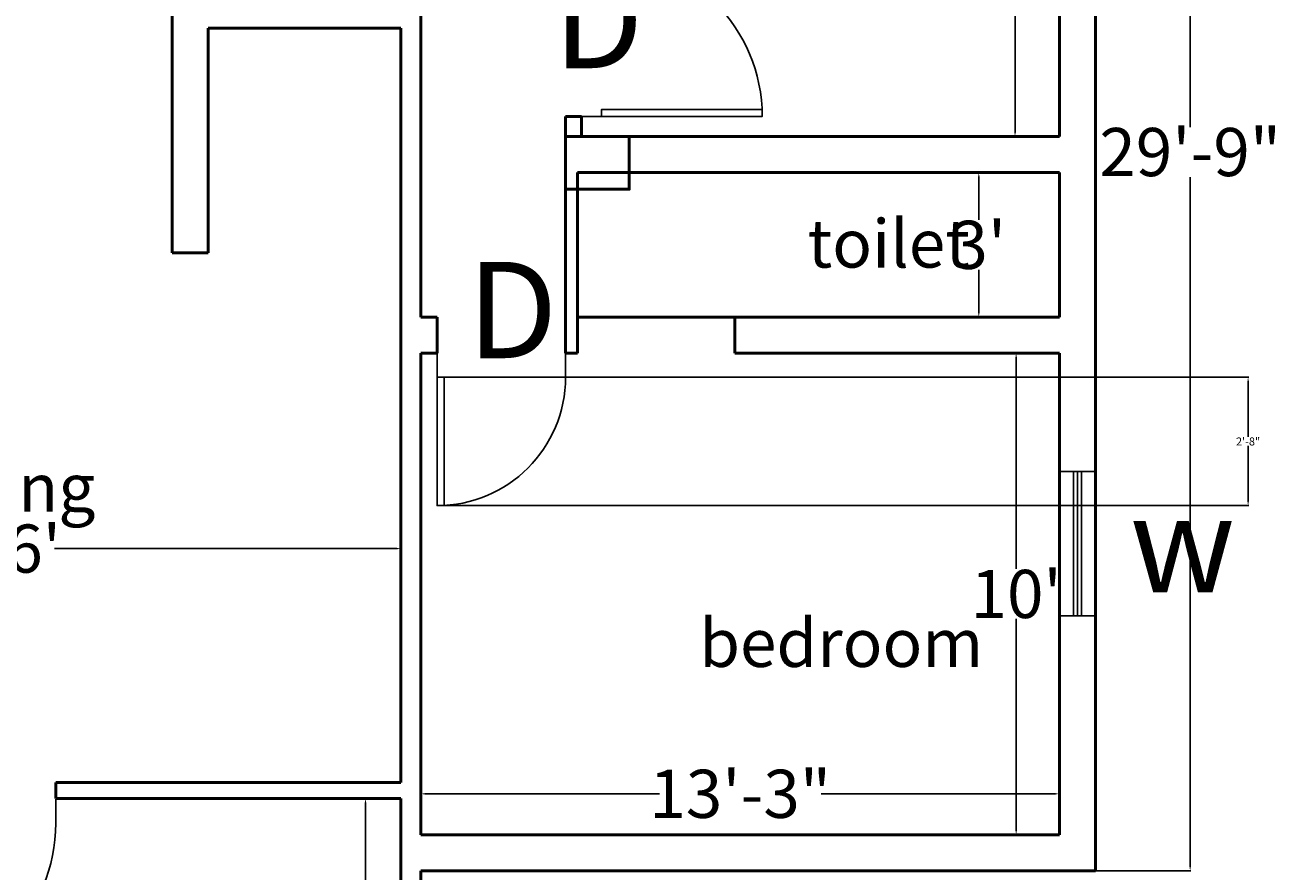
# Model space of a CAD drawing. Units: inches. Extents: x 409 to 7572, y 7 to 725.
# Tile 32 of 38: x 5952 to 6263, y 315 to 526. Entities that reach past the tile are written whole.
import ezdxf

# ---------------------------------------------------------------- set-up
doc = ezdxf.new("R2010")
doc.units = ezdxf.units.IN
doc.header["$MEASUREMENT"] = 0
for name, color, linetype, lineweight in [('A-ANNO-DIMS', 2, 'Continuous', 18), ('A-ANNO-SYMB', 3, 'Continuous', 25), ('A-AREA-IDEN', 7, 'Continuous', 25), ('A-DOOR', 3, 'Continuous', 25), ('A-GLAZ', 4, 'Continuous', 25), ('A-WALL', 7, 'Continuous', 50)]:
    doc.layers.add(name, color=color, linetype=linetype, lineweight=lineweight)
doc.styles.get("Standard").update_dxf_attribs({"font": 'arial.ttf'})
doc.dimstyles.get("Standard").update_dxf_attribs({"dimtxt": 2, "dimasz": 1, "dimexe": 0.18, "dimexo": 0.0625, "dimgap": 0.09, "dimtad": 0, "dimtih": 1, "dimtoh": 1, "dimdec": 0, "dimzin": 0, "dimdsep": 46, "dimlunit": 3, "dimtxsty": 'Standard', "dimcen": 0.09, "dimadec": 0, "dimazin": 0, "dimtfac": 1, "dimtdec": 0, "dimtofl": 0, "dimtmove": 0, "dimatfit": 3, "dimfxl": 1, "dimtolj": 1, "dimtzin": 0, "dimarcsym": 0})

# ---------------------------------------------------------------- blocks, each defined once
blk = doc.blocks.new('*U5')
for p, q in [((0, 0), (0, 6)), ((40, 0), (40, 6))]:
    blk.add_line(p, q)
blk.add_lwpolyline([(0, 0), (0, -40), (1.75, -40), (1.75, 0)], close=True)
blk.add_arc((0, 0), 40, 270, 0)
blk = doc.blocks.new('*U6')
for p, q in [((0, 0), (0, -6)), ((-40, 0), (-40, -6))]:
    blk.add_line(p, q)
blk.add_lwpolyline([(0, 0), (0, 40), (-1.75, 40), (-1.75, 0)], close=True)
blk.add_arc((0, 0), 40, 90, 180)
blk = doc.blocks.new('*U7')
for p, q in [((0, 0), (0, 6)), ((32, 0), (32, 6))]:
    blk.add_line(p, q)
blk.add_lwpolyline([(0, 0), (0, -32), (1.75, -32), (1.75, 0)], close=True)
blk.add_arc((0, 0), 32, 270, 0)
blk = doc.blocks.new('*D130')
at = {"layer": 'A-ANNO-DIMS', "color": 0, "lineweight": -2, "transparency": 16777216}
for p, q in [((6209.72, 618.53), (6198.55, 618.53)), ((6198.73, 617.53), (6198.73, 564.75)), ((6198.73, 499.53), (6198.73, 552.31)), ((6209.72, 498.53), (6198.55, 498.53))]:
    blk.add_line(p, q, dxfattribs=at)
at = {"layer": 'A-ANNO-DIMS', "color": 0, "transparency": 16777216}
for points in [[(6198.57, 617.53), (6198.9, 617.53), (6198.73, 618.53)], [(6198.57, 499.53), (6198.9, 499.53), (6198.73, 498.53)]]:
    blk.add_solid(points, dxfattribs=at)
at = {"layer": 'DEFPOINTS', "color": 0, "transparency": 16777216}
for p in [(6198.73, 618.53), (6209.78, 618.53), (6209.78, 498.53)]:
    blk.add_point(p, dxfattribs=at)
at = {"layer": 'A-ANNO-DIMS', "color": 0, "transparency": 16777216, "insert": (6198.73, 558.53), "char_height": 2, "attachment_point": 5}
blk.add_mtext("\\A1;{\\H6x;10'}", dxfattribs=at)
blk = doc.blocks.new('*D131')
at = {"layer": 'A-ANNO-DIMS', "color": 0, "lineweight": -2, "transparency": 16777216}
for p, q in [((6209.72, 444.53), (6198.84, 444.53)), ((6199.02, 443.53), (6199.02, 390.75)), ((6199.02, 325.53), (6199.02, 378.31)), ((6209.72, 324.53), (6198.84, 324.53))]:
    blk.add_line(p, q, dxfattribs=at)
at = {"layer": 'A-ANNO-DIMS', "color": 0, "transparency": 16777216}
for points in [[(6198.85, 443.53), (6199.18, 443.53), (6199.02, 444.53)], [(6198.85, 325.53), (6199.18, 325.53), (6199.02, 324.53)]]:
    blk.add_solid(points, dxfattribs=at)
at = {"layer": 'DEFPOINTS', "color": 0, "transparency": 16777216}
for p in [(6199.02, 444.53), (6209.78, 444.53), (6209.78, 324.53)]:
    blk.add_point(p, dxfattribs=at)
at = {"layer": 'A-ANNO-DIMS', "color": 0, "transparency": 16777216, "insert": (6199.02, 384.53), "char_height": 2, "attachment_point": 5}
blk.add_mtext("\\A1;{\\H6x;10'}", dxfattribs=at)
blk = doc.blocks.new('*D122')
at = {"layer": 'A-ANNO-DIMS', "color": 0, "lineweight": -2, "transparency": 16777216}
for p, q in [((6050.78, 324.59), (6050.78, 334.9)), ((6051.78, 334.72), (6110.15, 334.72)), ((6208.78, 334.72), (6150.42, 334.72)), ((6209.78, 324.59), (6209.78, 334.9))]:
    blk.add_line(p, q, dxfattribs=at)
at = {"layer": 'A-ANNO-DIMS', "color": 0, "transparency": 16777216}
for points in [[(6051.78, 334.88), (6051.78, 334.55), (6050.78, 334.72)], [(6208.78, 334.88), (6208.78, 334.55), (6209.78, 334.72)]]:
    blk.add_solid(points, dxfattribs=at)
at = {"layer": 'DEFPOINTS', "color": 0, "transparency": 16777216}
for p in [(6050.78, 334.72), (6050.78, 324.53), (6209.78, 324.53)]:
    blk.add_point(p, dxfattribs=at)
at = {"layer": 'A-ANNO-DIMS', "color": 0, "transparency": 16777216, "insert": (6130.28, 334.72), "char_height": 2, "attachment_point": 5}
blk.add_mtext('\\A1;{\\H6x;13\'-3"}', dxfattribs=at)
blk = doc.blocks.new('*D123')
at = {"layer": 'A-ANNO-DIMS', "color": 0, "lineweight": -2, "transparency": 16777216}
for p, q in [((6045.72, 333.53), (6036.79, 333.53)), ((6036.97, 332.53), (6036.97, 255.65)), ((6036.97, 166.53), (6036.97, 243.42)), ((6045.72, 165.53), (6036.79, 165.53))]:
    blk.add_line(p, q, dxfattribs=at)
at = {"layer": 'A-ANNO-DIMS', "color": 0, "transparency": 16777216}
for points in [[(6036.8, 332.53), (6037.14, 332.53), (6036.97, 333.53)], [(6036.8, 166.53), (6037.14, 166.53), (6036.97, 165.53)]]:
    blk.add_solid(points, dxfattribs=at)
at = {"layer": 'DEFPOINTS', "color": 0, "transparency": 16777216}
for p in [(6045.78, 333.53), (6036.97, 165.53), (6045.78, 165.53)]:
    blk.add_point(p, dxfattribs=at)
at = {"layer": 'A-ANNO-DIMS', "color": 0, "transparency": 16777216, "insert": (6036.97, 249.53), "char_height": 2, "attachment_point": 5}
blk.add_mtext("\\A1;{\\H6x;14'}", dxfattribs=at)
blk = doc.blocks.new('*D136')
at = {"layer": 'A-ANNO-DIMS', "color": 0, "lineweight": -2, "transparency": 16777216}
for p, q in [((5853.78, 403.47), (5853.78, 395.65)), ((6045.78, 403.47), (6045.78, 395.65)), ((5854.78, 395.83), (5940.08, 395.83)), ((6044.78, 395.83), (5959.49, 395.83))]:
    blk.add_line(p, q, dxfattribs=at)
at = {"layer": 'A-ANNO-DIMS', "color": 0, "transparency": 16777216}
for points in [[(5854.78, 396), (5854.78, 395.66), (5853.78, 395.83)], [(6044.78, 396), (6044.78, 395.66), (6045.78, 395.83)]]:
    blk.add_solid(points, dxfattribs=at)
at = {"layer": 'DEFPOINTS', "color": 0, "transparency": 16777216}
for p in [(5853.78, 403.53), (6045.78, 403.53), (6045.78, 395.83)]:
    blk.add_point(p, dxfattribs=at)
at = {"layer": 'A-ANNO-DIMS', "color": 0, "transparency": 16777216, "insert": (5949.78, 395.83), "char_height": 2, "attachment_point": 5}
blk.add_mtext("\\A1;{\\H6x;16'}", dxfattribs=at)
blk = doc.blocks.new('*D144')
at = {"layer": 'A-ANNO-DIMS', "color": 0, "lineweight": -2, "transparency": 16777216}
for p, q in [((6209.72, 489.53), (6189.53, 489.53)), ((6189.71, 488.53), (6189.71, 477.75)), ((6189.71, 454.53), (6189.71, 465.31)), ((6209.72, 453.53), (6189.53, 453.53))]:
    blk.add_line(p, q, dxfattribs=at)
at = {"layer": 'A-ANNO-DIMS', "color": 0, "transparency": 16777216}
for points in [[(6189.54, 488.53), (6189.88, 488.53), (6189.71, 489.53)], [(6189.54, 454.53), (6189.88, 454.53), (6189.71, 453.53)]]:
    blk.add_solid(points, dxfattribs=at)
at = {"layer": 'DEFPOINTS', "color": 0, "transparency": 16777216}
for p in [(6209.78, 489.53), (6189.71, 453.53), (6209.78, 453.53)]:
    blk.add_point(p, dxfattribs=at)
at = {"layer": 'A-ANNO-DIMS', "color": 0, "transparency": 16777216, "insert": (6189.71, 471.53), "char_height": 2, "attachment_point": 5}
blk.add_mtext("\\A1;{\\H6x;3'}", dxfattribs=at)
blk = doc.blocks.new('*D148')
at = {"layer": 'A-ANNO-DIMS', "color": 0, "lineweight": -2, "transparency": 16777216}
for p, q in [((6218.85, 672.53), (6242.53, 672.53)), ((6242.35, 671.53), (6242.35, 500.86)), ((6242.35, 316.53), (6242.35, 488.43)), ((6218.85, 315.53), (6242.53, 315.53))]:
    blk.add_line(p, q, dxfattribs=at)
at = {"layer": 'A-ANNO-DIMS', "color": 0, "transparency": 16777216}
for points in [[(6242.18, 671.53), (6242.52, 671.53), (6242.35, 672.53)], [(6242.18, 316.53), (6242.52, 316.53), (6242.35, 315.53)]]:
    blk.add_solid(points, dxfattribs=at)
at = {"layer": 'DEFPOINTS', "color": 0, "transparency": 16777216}
for p in [(6218.78, 672.53), (6242.35, 672.53), (6218.78, 315.53)]:
    blk.add_point(p, dxfattribs=at)
at = {"layer": 'A-ANNO-DIMS', "color": 0, "transparency": 16777216, "insert": (6242.35, 494.65), "char_height": 2, "attachment_point": 5}
blk.add_mtext('\\A1;{\\H6x;29\'-9"}', dxfattribs=at)
blk = doc.blocks.new('WIN-36')
for p, q in [((1699.82, 514.65), (1699.82, 478.65)), ((1700.82, 514.65), (1700.82, 478.65)), ((1701.82, 514.65), (1701.82, 478.65))]:
    blk.add_line(p, q)
blk.add_lwpolyline([(1705.32, 514.65), (1705.32, 478.65), (1696.32, 478.65), (1696.32, 514.65)], close=True)
blk = doc.blocks.new('*D195')
at = {"layer": 'A-ANNO-DIMS', "color": 0, "lineweight": -2, "transparency": 16777216}
for p, q in [((6054.85, 438.53), (6256.96, 438.53)), ((6256.78, 437.53), (6256.78, 423.64)), ((6256.78, 407.53), (6256.78, 421.42)), ((6054.85, 406.53), (6256.96, 406.53))]:
    blk.add_line(p, q, dxfattribs=at)
at = {"layer": 'A-ANNO-DIMS', "color": 0, "transparency": 16777216}
for points in [[(6256.62, 437.53), (6256.95, 437.53), (6256.78, 438.53)], [(6256.62, 407.53), (6256.95, 407.53), (6256.78, 406.53)]]:
    blk.add_solid(points, dxfattribs=at)
at = {"layer": 'DEFPOINTS', "color": 0, "transparency": 16777216}
for p in [(6054.78, 438.53), (6054.78, 406.53), (6256.78, 406.53)]:
    blk.add_point(p, dxfattribs=at)
at = {"layer": 'A-ANNO-DIMS', "color": 0, "transparency": 16777216, "insert": (6256.78, 422.53), "char_height": 2, "attachment_point": 5}
blk.add_mtext('\\A1;2\'-8"', dxfattribs=at)

msp = doc.modelspace()

# ---------------------------------------------------------------- linework, layer by layer
at = {"layer": 'A-WALL'}
for p, q in [((6218.78, 315.53), (6218.78, 672.53)), ((6209.78, 498.53), (6209.78, 618.53)), ((6050.78, 534.53), (6050.78, 453.53)), ((6045.78, 525.53), (5997.78, 525.53)), ((5997.78, 525.53), (5997.78, 469.53)), ((6045.78, 525.53), (6045.78, 337.53)), ((6086.78, 498.53), (6086.78, 503.53)), ((6086.78, 503.53), (6090.78, 503.53)), ((6090.78, 503.53), (6090.78, 498.53)), ((6209.78, 498.53), (6086.78, 498.53)), ((6086.78, 498.53), (6086.78, 444.53)), ((6045.78, 489.53), (6045.78, 337.53)), ((6209.78, 489.53), (6089.78, 489.53)), ((6089.78, 489.53), (6089.78, 444.53)), ((6209.78, 453.53), (6209.78, 489.53)), ((5988.78, 469.53), (5997.78, 469.53)), ((6054.78, 453.53), (6050.78, 453.53)), ((6054.78, 453.53), (6054.78, 444.53)), ((6209.78, 453.53), (6089.78, 453.53)), ((6128.98, 453.53), (6128.98, 444.53)), ((6054.78, 444.53), (6050.78, 444.53)), ((6050.78, 444.53), (6050.78, 324.53)), ((6089.78, 444.53), (6086.78, 444.53)), ((6089.78, 444.53), (6086.78, 444.53)), ((6209.78, 444.53), (6128.98, 444.53)), ((6209.78, 324.53), (6209.78, 444.53)), ((5959.84, 337.53), (6045.78, 337.53)), ((5959.84, 337.53), (5959.84, 333.53)), ((5959.84, 333.53), (6045.78, 333.53)), ((6045.78, 333.53), (6045.78, 165.53)), ((6045.78, 333.53), (6045.78, 165.53)), ((6209.78, 324.53), (6050.78, 324.53)), ((6218.78, 315.53), (6050.78, 315.53)), ((6050.78, 315.53), (6050.78, 165.53))]:
    msp.add_line(p, q, dxfattribs=at)
msp.add_lwpolyline([(5988.78, 594.53), (5988.78, 525.53), (5988.78, 469.53)], dxfattribs=at)
msp.add_lwpolyline([(6086.78, 498.53), (6102.65, 498.53), (6102.65, 485.36), (6086.78, 485.36)], close=True, dxfattribs=at)

# ---------------------------------------------------------------- block references
at = {"layer": 'A-DOOR', "rotation": 270}
msp.add_blockref('*U6', (6095.78, 503.53), dxfattribs=at)
at = {"layer": 'A-DOOR'}
for name, p in [('*U7', (6054.78, 438.53)), ('*U5', (5919.84, 327.37))]:
    msp.add_blockref(name, p, dxfattribs=at)
at = {"layer": 'A-GLAZ'}
msp.add_blockref('WIN-36', (4513.46, -99.57), dxfattribs=at)

# ---------------------------------------------------------------- texts
at = {"layer": 'A-ANNO-SYMB', "char_height": 24, "attachment_point": 1}
for s, width, insert in [('D', 19.1972, (6083.71, 539.54)), ('D', 19.1972, (6062.28, 467.28)), ('w', 18.2582, (6227.32, 408.94))]:
    msp.add_mtext_dynamic_manual_height_columns(s, width=width, gutter_width=1, heights=[0], dxfattribs=dict(at, insert=insert))
at = {"layer": 'A-AREA-IDEN', "char_height": 12, "attachment_point": 1}
for s, width, insert in [('toilet', 49.2946, (6147.04, 477.86)), ('Dining ', 67.5069, (5920.22, 417.03)), ('bedroom', 40.9017, (6120.12, 378.34))]:
    msp.add_mtext_dynamic_manual_height_columns(s, width=width, gutter_width=1, heights=[0], dxfattribs=dict(at, insert=insert))

# ---------------------------------------------------------------- dimensions: what is measured, and where the dimension line sits
at = {"layer": 'A-ANNO-DIMS'}
dim = msp.add_linear_dim(base=(6242.35, 672.53), p1=(6218.78, 315.53), p2=(6218.78, 672.53), angle=90, text='{\\H6x;<>}', dimstyle='Standard', override={"dimclrd": 0, "dimclre": 0, "dimclrt": 0}, dxfattribs=at)
dim.commit()
dim.dimension.update_dxf_attribs({"geometry": '*D148', "text_midpoint": (6242.35, 494.65), "dimtype": 160})
for base, p1, p2, picture, middle in [((6198.73, 618.53), (6209.78, 498.53), (6209.78, 618.53), '*D130', (6198.73, 558.53)), ((6189.71, 453.53), (6209.78, 489.53), (6209.78, 453.53), '*D144', (6189.71, 471.53)), ((6199.02, 444.53), (6209.78, 324.53), (6209.78, 444.53), '*D131', (6199.02, 384.53)), ((6036.97, 165.53), (6045.78, 333.53), (6045.78, 165.53), '*D123', (6036.97, 249.53))]:
    dim = msp.add_linear_dim(base=base, p1=p1, p2=p2, angle=90, text='{\\H6x;<>}', dimstyle='Standard', override={"dimclrd": 0, "dimclre": 0, "dimclrt": 0}, dxfattribs=at)
    dim.commit()
    dim.dimension.update_dxf_attribs({"geometry": picture, "text_midpoint": middle})
dim = msp.add_linear_dim(base=(6256.78, 406.53), p1=(6054.78, 438.53), p2=(6054.78, 406.53), angle=90, dimstyle='Standard', override={"dimdec": 1, "dimlfac": 1, "dimrnd": 0, "dimzin": 1, "dimdsep": 46, "dimlunit": 4, "dimfrac": 2}, dxfattribs=at)
dim.commit()
dim.dimension.update_dxf_attribs({"geometry": '*D195', "text_midpoint": (6256.78, 422.53)})
dim = msp.add_linear_dim(base=(6045.78, 395.83), p1=(5853.78, 403.53), p2=(6045.78, 403.53), text='{\\H6x;<>}', dimstyle='Standard', override={"dimclrd": 0, "dimclre": 0, "dimclrt": 0}, dxfattribs=at)
dim.commit()
dim.dimension.update_dxf_attribs({"geometry": '*D136', "text_midpoint": (5949.78, 395.83), "dimtype": 160})
dim = msp.add_linear_dim(base=(6050.78, 334.72), p1=(6209.78, 324.53), p2=(6050.78, 324.53), text='{\\H6x;<>}', dimstyle='Standard', override={"dimclrd": 0, "dimclre": 0, "dimclrt": 0}, dxfattribs=at)
dim.commit()
dim.dimension.update_dxf_attribs({"geometry": '*D122', "text_midpoint": (6130.28, 334.72)})

doc.saveas('drawing.dxf')
